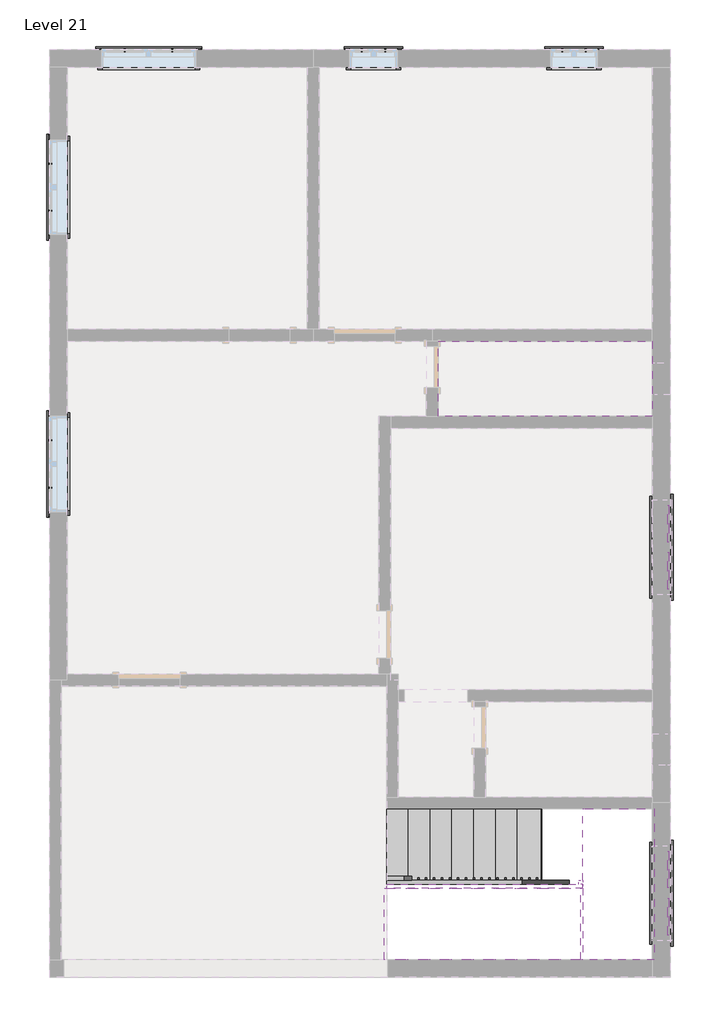
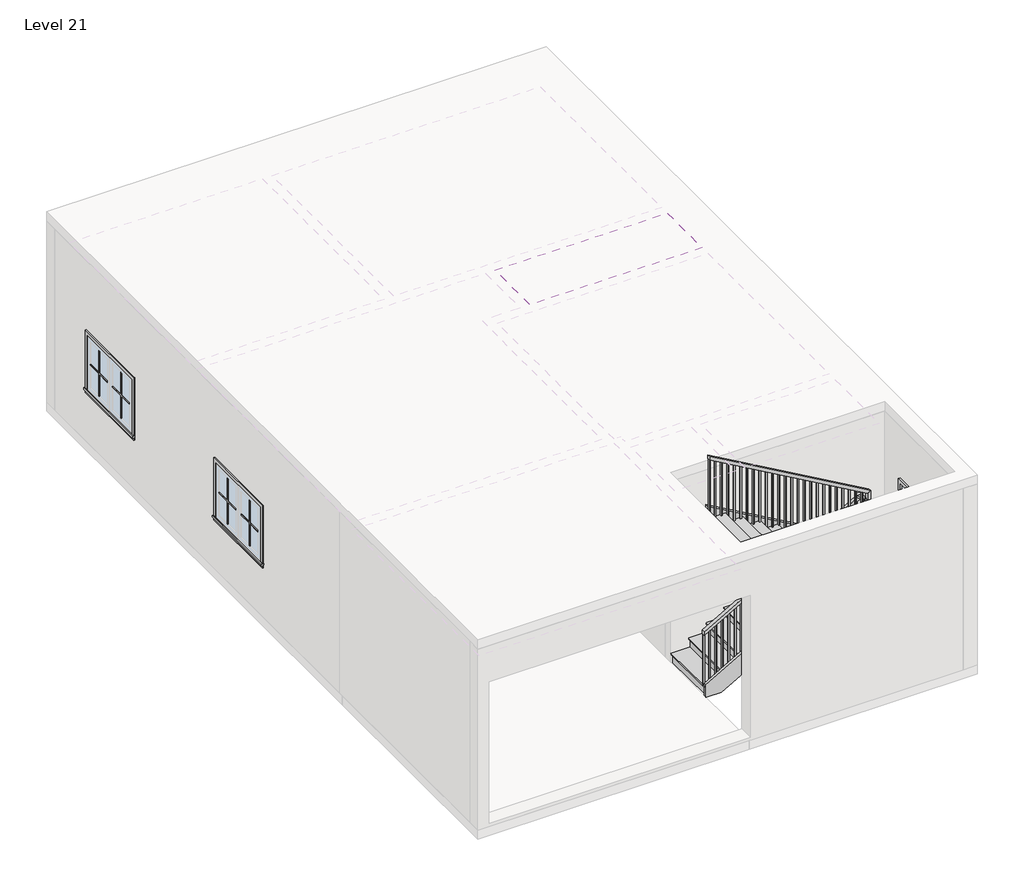
# One storey, part 2 of 2: 44 proxies, 3 members, 2 stair flights, 1 covering, 1 railing, 1 slab.
"""IFC4 building model written with IfcOpenShell, lengths in millimetres."""

from ifc_helpers import new_model, si_unit, frame, origin, place, context, project, spatial, polyline, outline, extrude, faceted_brep, transform, mapped, element, save
from components import muntin_pattern_2x2_muntin_pattern_2x2_2357e71d, muntin_pattern_2x2_muntin_pattern_2x2_302d8f29, muntin_pattern_2x2_muntin_pattern_2x2_53152e2c, muntin_pattern_2x2_muntin_pattern_2x2_e8f3e573, trim_window_exterior_flat_with_sill_c4e67c73, trim_window_exterior_flat_with_sill_a665a915, trim_window_interior_flat_picture_frame_cf1733af, trim_window_interior_flat_picture_frame_d485c387, non_monolithic_landing_5db28acc, stair_flight_6ff81285, stair_flight_de92f90a

model = new_model("IFC4")

# Units and contexts
model_context = context("Model", 3, world=origin())
ifc_project = project(units=[si_unit("LENGTHUNIT", "METRE", prefix="MILLI")], contexts=[model_context])

# Site, building, storey
site = spatial("IfcSite", under=ifc_project)
building = spatial("IfcBuilding", under=site)
storey = spatial("IfcBuildingStorey", under=building, Name="Level 21", Elevation=16002.0)

# Proxies
placement = place(None, origin())
muntin_pattern_2x2_muntin_pattern_2x2_shape = muntin_pattern_2x2_muntin_pattern_2x2_2357e71d(model_context)
element("IfcBuildingElementProxy", 1, Name="Muntin Pattern_2x2 : Muntin Pattern_2x2", ObjectType="Muntin Pattern_2x2 : Muntin Pattern_2x2", at=placement, inside=storey, context=model_context, shape_type="MappedRepresentation", body=[
    mapped(muntin_pattern_2x2_muntin_pattern_2x2_shape, transform((-4942.3279463, 5897.3080275, 16986.25), x_axis=(1.0, 0.0, 0.0), y_axis=(0.0, 1.0, 0.0), z_axis=(0.0, 0.0, 1.0))),
])
element("IfcBuildingElementProxy", 2, Name="Muntin Pattern_2x2 : Muntin Pattern_2x2", ObjectType="Muntin Pattern_2x2 : Muntin Pattern_2x2", at=placement, inside=storey, context=model_context, shape_type="MappedRepresentation", body=[
    mapped(muntin_pattern_2x2_muntin_pattern_2x2_shape, transform((-5899.5904463, 3838.3205275, 16986.25), x_axis=(0.0, 1.0, 0.0), y_axis=(-1.0, 0.0, 0.0), z_axis=(0.0, 0.0, 1.0))),
])
element("IfcBuildingElementProxy", 3, Name="Muntin Pattern_2x2 : Muntin Pattern_2x2", ObjectType="Muntin Pattern_2x2 : Muntin Pattern_2x2", at=placement, inside=storey, context=model_context, shape_type="MappedRepresentation", body=[
    mapped(muntin_pattern_2x2_muntin_pattern_2x2_shape, transform((-5899.5904463, 293.4330275, 16986.25), x_axis=(0.0, 1.0, 0.0), y_axis=(-1.0, 0.0, 0.0), z_axis=(0.0, 0.0, 1.0))),
])
element("IfcBuildingElementProxy", 4, Name="Muntin Pattern_2x2 : Muntin Pattern_2x2", ObjectType="Muntin Pattern_2x2 : Muntin Pattern_2x2", at=placement, inside=storey, context=model_context, shape_type="MappedRepresentation", body=[
    mapped(muntin_pattern_2x2_muntin_pattern_2x2_shape, transform((2031.5595537, -166.9419725, 17291.05), x_axis=(0.0, -1.0, 0.0), y_axis=(1.0, 0.0, 0.0), z_axis=(0.0, 0.0, 1.0))),
])
element("IfcBuildingElementProxy", 5, Name="Muntin Pattern_2x2 : Muntin Pattern_2x2", ObjectType="Muntin Pattern_2x2 : Muntin Pattern_2x2", at=placement, inside=storey, context=model_context, shape_type="MappedRepresentation", body=[
    mapped(muntin_pattern_2x2_muntin_pattern_2x2_shape, transform((2031.5595537, -4599.2419725, 17291.05), x_axis=(0.0, -1.0, 0.0), y_axis=(1.0, 0.0, 0.0), z_axis=(0.0, 0.0, 1.0))),
])
element("IfcBuildingElementProxy", 6, Name="Muntin Pattern_2x2 : Muntin Pattern_2x2", ObjectType="Muntin Pattern_2x2 : Muntin Pattern_2x2", at=placement, inside=storey, context=model_context, shape_type="MappedRepresentation", body=[
    mapped(muntin_pattern_2x2_muntin_pattern_2x2_shape, transform((-4942.3279463, 5897.3080275, 16986.25), x_axis=(1.0, 0.0, 0.0), y_axis=(0.0, 1.0, 0.0), z_axis=(0.0, 0.0, 1.0))),
])
element("IfcBuildingElementProxy", 7, Name="Muntin Pattern_2x2 : Muntin Pattern_2x2", ObjectType="Muntin Pattern_2x2 : Muntin Pattern_2x2", at=placement, inside=storey, context=model_context, shape_type="MappedRepresentation", body=[
    mapped(muntin_pattern_2x2_muntin_pattern_2x2_shape, transform((2031.5595537, -4599.2419725, 17291.05), x_axis=(0.0, -1.0, 0.0), y_axis=(1.0, 0.0, 0.0), z_axis=(0.0, 0.0, 1.0))),
])
muntin_pattern_2x2_muntin_pattern_2x2_2_shape = muntin_pattern_2x2_muntin_pattern_2x2_302d8f29(model_context)
element("IfcBuildingElementProxy", 8, Name="Muntin Pattern_2x2 : Muntin Pattern_2x2", ObjectType="Muntin Pattern_2x2 : Muntin Pattern_2x2", at=placement, inside=storey, context=model_context, shape_type="MappedRepresentation", body=[
    mapped(muntin_pattern_2x2_muntin_pattern_2x2_2_shape, transform((-4335.9029463, 5897.3080275, 16986.25), x_axis=(-1.0, 0.0, 0.0), y_axis=(0.0, -1.0, 0.0), z_axis=(0.0, 0.0, 1.0))),
])
element("IfcBuildingElementProxy", 9, Name="Muntin Pattern_2x2 : Muntin Pattern_2x2", ObjectType="Muntin Pattern_2x2 : Muntin Pattern_2x2", at=placement, inside=storey, context=model_context, shape_type="MappedRepresentation", body=[
    mapped(muntin_pattern_2x2_muntin_pattern_2x2_2_shape, transform((-5899.5904463, 4444.7455275, 16986.25), x_axis=(0.0, -1.0, 0.0), y_axis=(1.0, 0.0, 0.0), z_axis=(0.0, 0.0, 1.0))),
])
element("IfcBuildingElementProxy", 10, Name="Muntin Pattern_2x2 : Muntin Pattern_2x2", ObjectType="Muntin Pattern_2x2 : Muntin Pattern_2x2", at=placement, inside=storey, context=model_context, shape_type="MappedRepresentation", body=[
    mapped(muntin_pattern_2x2_muntin_pattern_2x2_2_shape, transform((-5899.5904463, 899.8580275, 16986.25), x_axis=(0.0, -1.0, 0.0), y_axis=(1.0, 0.0, 0.0), z_axis=(0.0, 0.0, 1.0))),
])
element("IfcBuildingElementProxy", 11, Name="Muntin Pattern_2x2 : Muntin Pattern_2x2", ObjectType="Muntin Pattern_2x2 : Muntin Pattern_2x2", at=placement, inside=storey, context=model_context, shape_type="MappedRepresentation", body=[
    mapped(muntin_pattern_2x2_muntin_pattern_2x2_2_shape, transform((2031.5595537, -773.3669725, 17291.05), x_axis=(0.0, 1.0, 0.0), y_axis=(-1.0, 0.0, 0.0), z_axis=(0.0, 0.0, 1.0))),
])
element("IfcBuildingElementProxy", 12, Name="Muntin Pattern_2x2 : Muntin Pattern_2x2", ObjectType="Muntin Pattern_2x2 : Muntin Pattern_2x2", at=placement, inside=storey, context=model_context, shape_type="MappedRepresentation", body=[
    mapped(muntin_pattern_2x2_muntin_pattern_2x2_2_shape, transform((2031.5595537, -5205.6669725, 17291.05), x_axis=(0.0, 1.0, 0.0), y_axis=(-1.0, 0.0, 0.0), z_axis=(0.0, 0.0, 1.0))),
])
element("IfcBuildingElementProxy", 13, Name="Muntin Pattern_2x2 : Muntin Pattern_2x2", ObjectType="Muntin Pattern_2x2 : Muntin Pattern_2x2", at=placement, inside=storey, context=model_context, shape_type="MappedRepresentation", body=[
    mapped(muntin_pattern_2x2_muntin_pattern_2x2_2_shape, transform((-4335.9029463, 5897.3080275, 16986.25), x_axis=(-1.0, 0.0, 0.0), y_axis=(0.0, -1.0, 0.0), z_axis=(0.0, 0.0, 1.0))),
])
element("IfcBuildingElementProxy", 14, Name="Muntin Pattern_2x2 : Muntin Pattern_2x2", ObjectType="Muntin Pattern_2x2 : Muntin Pattern_2x2", at=placement, inside=storey, context=model_context, shape_type="MappedRepresentation", body=[
    mapped(muntin_pattern_2x2_muntin_pattern_2x2_2_shape, transform((2031.5595537, -5205.6669725, 17291.05), x_axis=(0.0, 1.0, 0.0), y_axis=(-1.0, 0.0, 0.0), z_axis=(0.0, 0.0, 1.0))),
])
muntin_pattern_2x2_muntin_pattern_2x2_3_shape = muntin_pattern_2x2_muntin_pattern_2x2_53152e2c(model_context)
element("IfcBuildingElementProxy", 15, Name="Muntin Pattern_2x2 : Muntin Pattern_2x2", ObjectType="Muntin Pattern_2x2 : Muntin Pattern_2x2", at=placement, inside=storey, context=model_context, shape_type="MappedRepresentation", body=[
    mapped(muntin_pattern_2x2_muntin_pattern_2x2_3_shape, transform((-1907.0279463, 5897.3080275, 16986.25), x_axis=(1.0, 0.0, 0.0), y_axis=(0.0, 1.0, 0.0), z_axis=(0.0, 0.0, 1.0))),
])
element("IfcBuildingElementProxy", 16, Name="Muntin Pattern_2x2 : Muntin Pattern_2x2", ObjectType="Muntin Pattern_2x2 : Muntin Pattern_2x2", at=placement, inside=storey, context=model_context, shape_type="MappedRepresentation", body=[
    mapped(muntin_pattern_2x2_muntin_pattern_2x2_3_shape, transform((658.3720537, 5897.3080275, 16986.25), x_axis=(1.0, 0.0, 0.0), y_axis=(0.0, 1.0, 0.0), z_axis=(0.0, 0.0, 1.0))),
])
element("IfcBuildingElementProxy", 17, Name="Muntin Pattern_2x2 : Muntin Pattern_2x2", ObjectType="Muntin Pattern_2x2 : Muntin Pattern_2x2", at=placement, inside=storey, context=model_context, shape_type="MappedRepresentation", body=[
    mapped(muntin_pattern_2x2_muntin_pattern_2x2_3_shape, transform((-1907.0279463, 5897.3080275, 16986.25), x_axis=(1.0, 0.0, 0.0), y_axis=(0.0, 1.0, 0.0), z_axis=(0.0, 0.0, 1.0))),
])
element("IfcBuildingElementProxy", 18, Name="Muntin Pattern_2x2 : Muntin Pattern_2x2", ObjectType="Muntin Pattern_2x2 : Muntin Pattern_2x2", at=placement, inside=storey, context=model_context, shape_type="MappedRepresentation", body=[
    mapped(muntin_pattern_2x2_muntin_pattern_2x2_3_shape, transform((658.3720537, 5897.3080275, 16986.25), x_axis=(1.0, 0.0, 0.0), y_axis=(0.0, 1.0, 0.0), z_axis=(0.0, 0.0, 1.0))),
])
muntin_pattern_2x2_muntin_pattern_2x2_4_shape = muntin_pattern_2x2_muntin_pattern_2x2_e8f3e573(model_context)
element("IfcBuildingElementProxy", 19, Name="Muntin Pattern_2x2 : Muntin Pattern_2x2", ObjectType="Muntin Pattern_2x2 : Muntin Pattern_2x2", at=placement, inside=storey, context=model_context, shape_type="MappedRepresentation", body=[
    mapped(muntin_pattern_2x2_muntin_pattern_2x2_4_shape, transform((-1605.4029463, 5897.3080275, 16986.25), x_axis=(-1.0, 0.0, 0.0), y_axis=(0.0, -1.0, 0.0), z_axis=(0.0, 0.0, 1.0))),
])
element("IfcBuildingElementProxy", 20, Name="Muntin Pattern_2x2 : Muntin Pattern_2x2", ObjectType="Muntin Pattern_2x2 : Muntin Pattern_2x2", at=placement, inside=storey, context=model_context, shape_type="MappedRepresentation", body=[
    mapped(muntin_pattern_2x2_muntin_pattern_2x2_4_shape, transform((959.9970537, 5897.3080275, 16986.25), x_axis=(-1.0, 0.0, 0.0), y_axis=(0.0, -1.0, 0.0), z_axis=(0.0, 0.0, 1.0))),
])
element("IfcBuildingElementProxy", 21, Name="Muntin Pattern_2x2 : Muntin Pattern_2x2", ObjectType="Muntin Pattern_2x2 : Muntin Pattern_2x2", at=placement, inside=storey, context=model_context, shape_type="MappedRepresentation", body=[
    mapped(muntin_pattern_2x2_muntin_pattern_2x2_4_shape, transform((-1605.4029463, 5897.3080275, 16986.25), x_axis=(-1.0, 0.0, 0.0), y_axis=(0.0, -1.0, 0.0), z_axis=(0.0, 0.0, 1.0))),
])
element("IfcBuildingElementProxy", 22, Name="Muntin Pattern_2x2 : Muntin Pattern_2x2", ObjectType="Muntin Pattern_2x2 : Muntin Pattern_2x2", at=placement, inside=storey, context=model_context, shape_type="MappedRepresentation", body=[
    mapped(muntin_pattern_2x2_muntin_pattern_2x2_4_shape, transform((959.9970537, 5897.3080275, 16986.25), x_axis=(-1.0, 0.0, 0.0), y_axis=(0.0, -1.0, 0.0), z_axis=(0.0, 0.0, 1.0))),
])
trim_window_exterior_flat_with_sill_shape = trim_window_exterior_flat_with_sill_c4e67c73(model_context)
element("IfcBuildingElementProxy", 23, Name="Trim-Window-Exterior-Flat : with Sill", ObjectType="Trim-Window-Exterior-Flat : with Sill", at=placement, inside=storey, context=model_context, shape_type="MappedRepresentation", body=[
    mapped(trim_window_exterior_flat_with_sill_shape, transform((-4639.1154463, 5906.8330275, 17830.8), x_axis=(-1.0, 0.0, 0.0), y_axis=(0.0, 0.0, 1.0), z_axis=(0.0, 1.0, 0.0))),
])
element("IfcBuildingElementProxy", 24, Name="Trim-Window-Exterior-Flat : with Sill", ObjectType="Trim-Window-Exterior-Flat : with Sill", at=placement, inside=storey, context=model_context, shape_type="MappedRepresentation", body=[
    mapped(trim_window_exterior_flat_with_sill_shape, transform((-5909.1154463, 4141.5330275, 17830.8), x_axis=(0.0, -1.0, 0.0), y_axis=(0.0, 0.0, 1.0), z_axis=(-1.0, 0.0, 0.0))),
])
element("IfcBuildingElementProxy", 25, Name="Trim-Window-Exterior-Flat : with Sill", ObjectType="Trim-Window-Exterior-Flat : with Sill", at=placement, inside=storey, context=model_context, shape_type="MappedRepresentation", body=[
    mapped(trim_window_exterior_flat_with_sill_shape, transform((-5909.1154463, 596.6455275, 17830.8), x_axis=(0.0, -1.0, 0.0), y_axis=(0.0, 0.0, 1.0), z_axis=(-1.0, 0.0, 0.0))),
])
element("IfcBuildingElementProxy", 26, Name="Trim-Window-Exterior-Flat : with Sill", ObjectType="Trim-Window-Exterior-Flat : with Sill", at=placement, inside=storey, context=model_context, shape_type="MappedRepresentation", body=[
    mapped(trim_window_exterior_flat_with_sill_shape, transform((2041.0845537, -470.1544725, 18135.6), x_axis=(0.0, 1.0, 0.0), y_axis=(0.0, 0.0, 1.0), z_axis=(1.0, 0.0, 0.0))),
])
element("IfcBuildingElementProxy", 27, Name="Trim-Window-Exterior-Flat : with Sill", ObjectType="Trim-Window-Exterior-Flat : with Sill", at=placement, inside=storey, context=model_context, shape_type="MappedRepresentation", body=[
    mapped(trim_window_exterior_flat_with_sill_shape, transform((2041.0845537, -4902.4544725, 18135.6), x_axis=(0.0, 1.0, 0.0), y_axis=(0.0, 0.0, 1.0), z_axis=(1.0, 0.0, 0.0))),
])
element("IfcBuildingElementProxy", 28, Name="Trim-Window-Exterior-Flat : with Sill", ObjectType="Trim-Window-Exterior-Flat : with Sill", at=placement, inside=storey, context=model_context, shape_type="MappedRepresentation", body=[
    mapped(trim_window_exterior_flat_with_sill_shape, transform((-4639.1154463, 5906.8330275, 17830.8), x_axis=(-1.0, 0.0, 0.0), y_axis=(0.0, 0.0, 1.0), z_axis=(0.0, 1.0, 0.0))),
])
element("IfcBuildingElementProxy", 29, Name="Trim-Window-Exterior-Flat : with Sill", ObjectType="Trim-Window-Exterior-Flat : with Sill", at=placement, inside=storey, context=model_context, shape_type="MappedRepresentation", body=[
    mapped(trim_window_exterior_flat_with_sill_shape, transform((2041.0845537, -4902.4544725, 18135.6), x_axis=(0.0, 1.0, 0.0), y_axis=(0.0, 0.0, 1.0), z_axis=(1.0, 0.0, 0.0))),
])
trim_window_exterior_flat_with_sill_2_shape = trim_window_exterior_flat_with_sill_a665a915(model_context)
element("IfcBuildingElementProxy", 30, Name="Trim-Window-Exterior-Flat : with Sill", ObjectType="Trim-Window-Exterior-Flat : with Sill", at=placement, inside=storey, context=model_context, shape_type="MappedRepresentation", body=[
    mapped(trim_window_exterior_flat_with_sill_2_shape, transform((-1756.2154463, 5906.8330275, 17830.8), x_axis=(-1.0, 0.0, 0.0), y_axis=(0.0, 0.0, 1.0), z_axis=(0.0, 1.0, 0.0))),
])
element("IfcBuildingElementProxy", 31, Name="Trim-Window-Exterior-Flat : with Sill", ObjectType="Trim-Window-Exterior-Flat : with Sill", at=placement, inside=storey, context=model_context, shape_type="MappedRepresentation", body=[
    mapped(trim_window_exterior_flat_with_sill_2_shape, transform((809.1845537, 5906.8330275, 17830.8), x_axis=(-1.0, 0.0, 0.0), y_axis=(0.0, 0.0, 1.0), z_axis=(0.0, 1.0, 0.0))),
])
element("IfcBuildingElementProxy", 32, Name="Trim-Window-Exterior-Flat : with Sill", ObjectType="Trim-Window-Exterior-Flat : with Sill", at=placement, inside=storey, context=model_context, shape_type="MappedRepresentation", body=[
    mapped(trim_window_exterior_flat_with_sill_2_shape, transform((-1756.2154463, 5906.8330275, 17830.8), x_axis=(-1.0, 0.0, 0.0), y_axis=(0.0, 0.0, 1.0), z_axis=(0.0, 1.0, 0.0))),
])
element("IfcBuildingElementProxy", 33, Name="Trim-Window-Exterior-Flat : with Sill", ObjectType="Trim-Window-Exterior-Flat : with Sill", at=placement, inside=storey, context=model_context, shape_type="MappedRepresentation", body=[
    mapped(trim_window_exterior_flat_with_sill_2_shape, transform((809.1845537, 5906.8330275, 17830.8), x_axis=(-1.0, 0.0, 0.0), y_axis=(0.0, 0.0, 1.0), z_axis=(0.0, 1.0, 0.0))),
])
trim_window_interior_flat_picture_frame_shape = trim_window_interior_flat_picture_frame_cf1733af(model_context)
element("IfcBuildingElementProxy", 34, Name="Trim-Window-Interior-Flat : Picture Frame", ObjectType="Trim-Window-Interior-Flat : Picture Frame", at=placement, inside=storey, context=model_context, shape_type="MappedRepresentation", body=[
    mapped(trim_window_interior_flat_picture_frame_shape, transform((-4639.1154463, 5678.2330275, 17830.8), x_axis=(1.0, 0.0, 0.0), y_axis=(0.0, 0.0, 1.0), z_axis=(0.0, -1.0, 0.0))),
])
element("IfcBuildingElementProxy", 35, Name="Trim-Window-Interior-Flat : Picture Frame", ObjectType="Trim-Window-Interior-Flat : Picture Frame", at=placement, inside=storey, context=model_context, shape_type="MappedRepresentation", body=[
    mapped(trim_window_interior_flat_picture_frame_shape, transform((-5680.5154463, 4141.5330275, 17830.8), x_axis=(0.0, 1.0, 0.0), y_axis=(0.0, 0.0, 1.0), z_axis=(1.0, 0.0, 0.0))),
])
element("IfcBuildingElementProxy", 36, Name="Trim-Window-Interior-Flat : Picture Frame", ObjectType="Trim-Window-Interior-Flat : Picture Frame", at=placement, inside=storey, context=model_context, shape_type="MappedRepresentation", body=[
    mapped(trim_window_interior_flat_picture_frame_shape, transform((-5680.5154463, 596.6455275, 17830.8), x_axis=(0.0, 1.0, 0.0), y_axis=(0.0, 0.0, 1.0), z_axis=(1.0, 0.0, 0.0))),
])
element("IfcBuildingElementProxy", 37, Name="Trim-Window-Interior-Flat : Picture Frame", ObjectType="Trim-Window-Interior-Flat : Picture Frame", at=placement, inside=storey, context=model_context, shape_type="MappedRepresentation", body=[
    mapped(trim_window_interior_flat_picture_frame_shape, transform((1812.4845537, -470.1544725, 18135.6), x_axis=(0.0, -1.0, 0.0), y_axis=(0.0, 0.0, 1.0), z_axis=(-1.0, 0.0, 0.0))),
])
element("IfcBuildingElementProxy", 38, Name="Trim-Window-Interior-Flat : Picture Frame", ObjectType="Trim-Window-Interior-Flat : Picture Frame", at=placement, inside=storey, context=model_context, shape_type="MappedRepresentation", body=[
    mapped(trim_window_interior_flat_picture_frame_shape, transform((1812.4845537, -4902.4544725, 18135.6), x_axis=(0.0, -1.0, 0.0), y_axis=(0.0, 0.0, 1.0), z_axis=(-1.0, 0.0, 0.0))),
])
element("IfcBuildingElementProxy", 39, Name="Trim-Window-Interior-Flat : Picture Frame", ObjectType="Trim-Window-Interior-Flat : Picture Frame", at=placement, inside=storey, context=model_context, shape_type="MappedRepresentation", body=[
    mapped(trim_window_interior_flat_picture_frame_shape, transform((-4639.1154463, 5678.2330275, 17830.8), x_axis=(1.0, 0.0, 0.0), y_axis=(0.0, 0.0, 1.0), z_axis=(0.0, -1.0, 0.0))),
])
element("IfcBuildingElementProxy", 40, Name="Trim-Window-Interior-Flat : Picture Frame", ObjectType="Trim-Window-Interior-Flat : Picture Frame", at=placement, inside=storey, context=model_context, shape_type="MappedRepresentation", body=[
    mapped(trim_window_interior_flat_picture_frame_shape, transform((1812.4845537, -4902.4544725, 18135.6), x_axis=(0.0, -1.0, 0.0), y_axis=(0.0, 0.0, 1.0), z_axis=(-1.0, 0.0, 0.0))),
])
trim_window_interior_flat_picture_frame_2_shape = trim_window_interior_flat_picture_frame_d485c387(model_context)
element("IfcBuildingElementProxy", 41, Name="Trim-Window-Interior-Flat : Picture Frame", ObjectType="Trim-Window-Interior-Flat : Picture Frame", at=placement, inside=storey, context=model_context, shape_type="MappedRepresentation", body=[
    mapped(trim_window_interior_flat_picture_frame_2_shape, transform((-1756.2154463, 5678.2330275, 17830.8), x_axis=(1.0, 0.0, 0.0), y_axis=(0.0, 0.0, 1.0), z_axis=(0.0, -1.0, 0.0))),
])
element("IfcBuildingElementProxy", 42, Name="Trim-Window-Interior-Flat : Picture Frame", ObjectType="Trim-Window-Interior-Flat : Picture Frame", at=placement, inside=storey, context=model_context, shape_type="MappedRepresentation", body=[
    mapped(trim_window_interior_flat_picture_frame_2_shape, transform((809.1845537, 5678.2330275, 17830.8), x_axis=(1.0, 0.0, 0.0), y_axis=(0.0, 0.0, 1.0), z_axis=(0.0, -1.0, 0.0))),
])
element("IfcBuildingElementProxy", 43, Name="Trim-Window-Interior-Flat : Picture Frame", ObjectType="Trim-Window-Interior-Flat : Picture Frame", at=placement, inside=storey, context=model_context, shape_type="MappedRepresentation", body=[
    mapped(trim_window_interior_flat_picture_frame_2_shape, transform((-1756.2154463, 5678.2330275, 17830.8), x_axis=(1.0, 0.0, 0.0), y_axis=(0.0, 0.0, 1.0), z_axis=(0.0, -1.0, 0.0))),
])
element("IfcBuildingElementProxy", 44, Name="Trim-Window-Interior-Flat : Picture Frame", ObjectType="Trim-Window-Interior-Flat : Picture Frame", at=placement, inside=storey, context=model_context, shape_type="MappedRepresentation", body=[
    mapped(trim_window_interior_flat_picture_frame_2_shape, transform((809.1845537, 5678.2330275, 17830.8), x_axis=(1.0, 0.0, 0.0), y_axis=(0.0, 0.0, 1.0), z_axis=(0.0, -1.0, 0.0))),
])

# Covering
element("IfcCovering", 45, ObjectType="2' x 4' ACT System", at=placement, inside=storey, context=model_context, shape_type="SweptSolid", body=[
    extrude(outline(polyline([(-930.7154463, 2171.4455275), (1812.4845537, 2171.4455275), (1812.4845537, 1206.2455275), (-930.7154463, 1206.2455275), (-930.7154463, 2171.4455275)])), frame((0.0, 0.0, 18745.2), z_axis=(0.0, 0.0, 1.0), x_axis=(1.0, 0.0, 0.0)), (0.0, 0.0, 1.0), 57.15),
])

# Members
element("IfcMember", 46, ObjectType="Stringer - 2\" Width", at=placement, inside=storey, context=model_context, shape_type="SweptSolid", body=[
    extrude(outline(polyline([(16211.0890626, -1591.1154463), (16002.0, -1591.1154463), (16002.0, -1342.8974141), (17270.924218, 872.6845537), (17622.1745172, 872.6845537), (16211.0890626, -1591.1154463)])), frame((0.0, -4788.1544725, 0.0), z_axis=(0.0, 1.0, 0.0), x_axis=(0.0, 0.0, 1.0)), (0.0, 0.0, 1.0), 50.8),
])
element("IfcMember", 47, ObjectType="Stringer - 2\" Width", at=placement, inside=storey, context=model_context, shape_type="SweptSolid", body=[
    extrude(outline(polyline([(17460.0387634, 923.4845537), (17811.2890626, 923.4845537), (19251.4690626, -1591.1154463), (18900.2187634, -1591.1154463), (17460.0387634, 923.4845537)])), frame((0.0, -4838.9544725, 0.0), z_axis=(0.0, 1.0, 0.0), x_axis=(0.0, 0.0, 1.0)), (0.0, 0.0, 1.0), 50.8),
])
element("IfcMember", 48, ObjectType="Stringer - 2\" Width", at=placement, inside=storey, context=model_context, shape_type="SweptSolid", body=[
    extrude(outline(polyline([(872.6845537, -4737.3544725), (923.4845537, -4737.3544725), (923.4845537, -4788.1544725), (872.6845537, -4788.1544725), (872.6845537, -4737.3544725)])), frame((0.0, 0.0, 17373.6), z_axis=(0.0, 0.0, 1.0), x_axis=(1.0, 0.0, 0.0)), (0.0, 0.0, 1.0), 304.8),
])

# Railing
element("IfcRailing", 49, ObjectType="Handrail - Rectangular", at=placement, inside=storey, context=model_context, shape_type="SolidModel", body=[
    faceted_brep([(-1591.1154463, -4686.5544725, 17076.42), (-1591.1154463, -4686.5544725, 17017.8782835), (-1591.1154463, -4737.3544725, 17017.8782835), (-1591.1154463, -4737.3544725, 17076.42), (847.2845537, -4686.5544725, 18472.9581818), (898.0845537, -4686.5544725, 18443.5110107), (898.0845537, -4737.3544725, 18443.5110107), (847.2845537, -4737.3544725, 18472.9581818), (847.2845537, -4686.5544725, 18516.6), (898.0845537, -4686.5544725, 18465.8), (898.0845537, -4737.3544725, 18465.8), (847.2845537, -4737.3544725, 18516.6), (974.2845537, -4686.5544725, 18516.6), (974.2845537, -4686.5544725, 18465.8), (923.4845537, -4737.3544725, 18465.8), (923.4845537, -4737.3544725, 18516.6), (974.2845537, -4813.5544725, 18516.6), (974.2845537, -4813.5544725, 18465.8), (923.4845537, -4813.5544725, 18465.8), (923.4845537, -4813.5544725, 18516.6), (974.2845537, -4838.9544725, 18516.6), (923.4845537, -4838.9544725, 18516.6), (923.4845537, -4889.7544725, 18465.8), (974.2845537, -4889.7544725, 18465.8)], [[[0, 1, 2, 3]], [[1, 0, 4, 5]], [[2, 1, 5, 6]], [[3, 2, 6, 7]], [[0, 3, 7, 4]], [[5, 4, 8, 9]], [[6, 5, 9, 10]], [[7, 6, 10, 11]], [[4, 7, 11, 8]], [[9, 8, 12, 13]], [[10, 9, 13, 14]], [[11, 10, 14, 15]], [[8, 11, 15, 12]], [[13, 12, 16, 17]], [[14, 13, 17, 18]], [[15, 14, 18, 19]], [[12, 15, 19, 16]], [[20, 21, 22, 23]], [[17, 16, 20, 23]], [[18, 17, 23, 22]], [[19, 18, 22, 21]], [[16, 19, 21, 20]]]),
    faceted_brep([(974.2845537, -4838.9544725, 18516.6), (974.2845537, -4889.7544725, 18465.8), (923.4845537, -4889.7544725, 18465.8), (923.4845537, -4838.9544725, 18516.6), (974.2845537, -4838.9544725, 18647.5254545), (923.4845537, -4838.9544725, 18618.0782835), (923.4845537, -4889.7544725, 18618.0782835), (974.2845537, -4889.7544725, 18647.5254545)], [[[0, 1, 2, 3]], [[4, 5, 6, 7]], [[1, 0, 4, 7]], [[2, 1, 7, 6]], [[3, 2, 6, 5]], [[0, 3, 5, 4]]]),
    faceted_brep([(974.2845537, -4889.7544725, 18647.5254545), (923.4845537, -4889.7544725, 18618.0782835), (923.4845537, -4838.9544725, 18618.0782835), (974.2845537, -4838.9544725, 18647.5254545), (-1591.1154463, -4889.7544725, 20116.8), (-1591.1154463, -4838.9544725, 20116.8), (-1591.1154463, -4838.9544725, 20058.2582835), (-1591.1154463, -4889.7544725, 20058.2582835)], [[[0, 1, 2, 3]], [[4, 5, 6, 7]], [[1, 0, 4, 7]], [[2, 1, 7, 6]], [[3, 2, 6, 5]], [[0, 3, 5, 4]]]),
    extrude(outline(polyline([(19994.6139653, -1479.9904463), (20005.5244198, -1499.0404463), (19042.38, -1499.0404463), (19042.38, -1479.9904463), (19994.6139653, -1479.9904463)])), frame((0.0, -4873.8794725, 0.0), z_axis=(0.0, 1.0, 0.0), x_axis=(0.0, 0.0, 1.0)), (0.0, 0.0, 1.0), 19.05),
    extrude(outline(polyline([(19936.4248744, -1378.3904463), (19947.3353289, -1397.4404463), (19042.38, -1397.4404463), (19042.38, -1378.3904463), (19936.4248744, -1378.3904463)])), frame((0.0, -4873.8794725, 0.0), z_axis=(0.0, 1.0, 0.0), x_axis=(0.0, 0.0, 1.0)), (0.0, 0.0, 1.0), 19.05),
    extrude(outline(polyline([(19878.2357835, -1276.7904463), (19889.146238, -1295.8404463), (18882.36, -1295.8404463), (18882.36, -1276.7904463), (19878.2357835, -1276.7904463)])), frame((0.0, -4873.8794725, 0.0), z_axis=(0.0, 1.0, 0.0), x_axis=(0.0, 0.0, 1.0)), (0.0, 0.0, 1.0), 19.05),
    extrude(outline(polyline([(19820.0466926, -1175.1904463), (19830.9571471, -1194.2404463), (18882.36, -1194.2404463), (18882.36, -1175.1904463), (19820.0466926, -1175.1904463)])), frame((0.0, -4873.8794725, 0.0), z_axis=(0.0, 1.0, 0.0), x_axis=(0.0, 0.0, 1.0)), (0.0, 0.0, 1.0), 19.05),
    extrude(outline(polyline([(19761.8576016, -1073.5904463), (19772.7680562, -1092.6404463), (18882.36, -1092.6404463), (18882.36, -1073.5904463), (19761.8576016, -1073.5904463)])), frame((0.0, -4873.8794725, 0.0), z_axis=(0.0, 1.0, 0.0), x_axis=(0.0, 0.0, 1.0)), (0.0, 0.0, 1.0), 19.05),
    extrude(outline(polyline([(19703.6685107, -971.9904463), (19714.5789653, -991.0404463), (18722.34, -991.0404463), (18722.34, -971.9904463), (19703.6685107, -971.9904463)])), frame((0.0, -4873.8794725, 0.0), z_axis=(0.0, 1.0, 0.0), x_axis=(0.0, 0.0, 1.0)), (0.0, 0.0, 1.0), 19.05),
    extrude(outline(polyline([(19645.4794198, -870.3904463), (19656.3898744, -889.4404463), (18722.34, -889.4404463), (18722.34, -870.3904463), (19645.4794198, -870.3904463)])), frame((0.0, -4873.8794725, 0.0), z_axis=(0.0, 1.0, 0.0), x_axis=(0.0, 0.0, 1.0)), (0.0, 0.0, 1.0), 19.05),
    extrude(outline(polyline([(19587.2903289, -768.7904463), (19598.2007835, -787.8404463), (18722.34, -787.8404463), (18722.34, -768.7904463), (19587.2903289, -768.7904463)])), frame((0.0, -4873.8794725, 0.0), z_axis=(0.0, 1.0, 0.0), x_axis=(0.0, 0.0, 1.0)), (0.0, 0.0, 1.0), 19.05),
    extrude(outline(polyline([(19529.101238, -667.1904463), (19540.0116926, -686.2404463), (18562.32, -686.2404463), (18562.32, -667.1904463), (19529.101238, -667.1904463)])), frame((0.0, -4873.8794725, 0.0), z_axis=(0.0, 1.0, 0.0), x_axis=(0.0, 0.0, 1.0)), (0.0, 0.0, 1.0), 19.05),
    extrude(outline(polyline([(19470.9121471, -565.5904463), (19481.8226016, -584.6404463), (18562.32, -584.6404463), (18562.32, -565.5904463), (19470.9121471, -565.5904463)])), frame((0.0, -4873.8794725, 0.0), z_axis=(0.0, 1.0, 0.0), x_axis=(0.0, 0.0, 1.0)), (0.0, 0.0, 1.0), 19.05),
    extrude(outline(polyline([(19412.7230562, -463.9904463), (19423.6335107, -483.0404463), (18562.32, -483.0404463), (18562.32, -463.9904463), (19412.7230562, -463.9904463)])), frame((0.0, -4873.8794725, 0.0), z_axis=(0.0, 1.0, 0.0), x_axis=(0.0, 0.0, 1.0)), (0.0, 0.0, 1.0), 19.05),
    extrude(outline(polyline([(19354.5339653, -362.3904463), (19365.4444198, -381.4404463), (18402.3, -381.4404463), (18402.3, -362.3904463), (19354.5339653, -362.3904463)])), frame((0.0, -4873.8794725, 0.0), z_axis=(0.0, 1.0, 0.0), x_axis=(0.0, 0.0, 1.0)), (0.0, 0.0, 1.0), 19.05),
    extrude(outline(polyline([(19296.3448744, -260.7904463), (19307.2553289, -279.8404463), (18402.3, -279.8404463), (18402.3, -260.7904463), (19296.3448744, -260.7904463)])), frame((0.0, -4873.8794725, 0.0), z_axis=(0.0, 1.0, 0.0), x_axis=(0.0, 0.0, 1.0)), (0.0, 0.0, 1.0), 19.05),
    extrude(outline(polyline([(19238.1557835, -159.1904463), (19249.066238, -178.2404463), (18242.28, -178.2404463), (18242.28, -159.1904463), (19238.1557835, -159.1904463)])), frame((0.0, -4873.8794725, 0.0), z_axis=(0.0, 1.0, 0.0), x_axis=(0.0, 0.0, 1.0)), (0.0, 0.0, 1.0), 19.05),
    extrude(outline(polyline([(19179.9666926, -57.5904463), (19190.8771471, -76.6404463), (18242.28, -76.6404463), (18242.28, -57.5904463), (19179.9666926, -57.5904463)])), frame((0.0, -4873.8794725, 0.0), z_axis=(0.0, 1.0, 0.0), x_axis=(0.0, 0.0, 1.0)), (0.0, 0.0, 1.0), 19.05),
    extrude(outline(polyline([(19121.7776016, 44.0095537), (19132.6880562, 24.9595537), (18242.28, 24.9595537), (18242.28, 44.0095537), (19121.7776016, 44.0095537)])), frame((0.0, -4873.8794725, 0.0), z_axis=(0.0, 1.0, 0.0), x_axis=(0.0, 0.0, 1.0)), (0.0, 0.0, 1.0), 19.05),
    extrude(outline(polyline([(19063.5885107, 145.6095537), (19074.4989653, 126.5595537), (18082.26, 126.5595537), (18082.26, 145.6095537), (19063.5885107, 145.6095537)])), frame((0.0, -4873.8794725, 0.0), z_axis=(0.0, 1.0, 0.0), x_axis=(0.0, 0.0, 1.0)), (0.0, 0.0, 1.0), 19.05),
    extrude(outline(polyline([(19005.3994198, 247.2095537), (19016.3098744, 228.1595537), (18082.26, 228.1595537), (18082.26, 247.2095537), (19005.3994198, 247.2095537)])), frame((0.0, -4873.8794725, 0.0), z_axis=(0.0, 1.0, 0.0), x_axis=(0.0, 0.0, 1.0)), (0.0, 0.0, 1.0), 19.05),
    extrude(outline(polyline([(18947.2103289, 348.8095537), (18958.1207835, 329.7595537), (18082.26, 329.7595537), (18082.26, 348.8095537), (18947.2103289, 348.8095537)])), frame((0.0, -4873.8794725, 0.0), z_axis=(0.0, 1.0, 0.0), x_axis=(0.0, 0.0, 1.0)), (0.0, 0.0, 1.0), 19.05),
    extrude(outline(polyline([(18889.021238, 450.4095537), (18899.9316926, 431.3595537), (17922.24, 431.3595537), (17922.24, 450.4095537), (18889.021238, 450.4095537)])), frame((0.0, -4873.8794725, 0.0), z_axis=(0.0, 1.0, 0.0), x_axis=(0.0, 0.0, 1.0)), (0.0, 0.0, 1.0), 19.05),
    extrude(outline(polyline([(18830.8321471, 552.0095537), (18841.7426016, 532.9595537), (17922.24, 532.9595537), (17922.24, 552.0095537), (18830.8321471, 552.0095537)])), frame((0.0, -4873.8794725, 0.0), z_axis=(0.0, 1.0, 0.0), x_axis=(0.0, 0.0, 1.0)), (0.0, 0.0, 1.0), 19.05),
    extrude(outline(polyline([(18772.6430562, 653.6095537), (18783.5535107, 634.5595537), (17922.24, 634.5595537), (17922.24, 653.6095537), (18772.6430562, 653.6095537)])), frame((0.0, -4873.8794725, 0.0), z_axis=(0.0, 1.0, 0.0), x_axis=(0.0, 0.0, 1.0)), (0.0, 0.0, 1.0), 19.05),
    extrude(outline(polyline([(18714.4539653, 755.2095537), (18725.3644198, 736.1595537), (17762.22, 736.1595537), (17762.22, 755.2095537), (18714.4539653, 755.2095537)])), frame((0.0, -4873.8794725, 0.0), z_axis=(0.0, 1.0, 0.0), x_axis=(0.0, 0.0, 1.0)), (0.0, 0.0, 1.0), 19.05),
    extrude(outline(polyline([(18656.2648744, 856.8095537), (18667.1753289, 837.7595537), (17762.22, 837.7595537), (17762.22, 856.8095537), (18656.2648744, 856.8095537)])), frame((0.0, -4873.8794725, 0.0), z_axis=(0.0, 1.0, 0.0), x_axis=(0.0, 0.0, 1.0)), (0.0, 0.0, 1.0), 19.05),
    extrude(outline(polyline([(939.3595537, -4804.0294725), (958.4095537, -4804.0294725), (958.4095537, -4823.0794725), (939.3595537, -4823.0794725), (939.3595537, -4804.0294725)])), frame((0.0, 0.0, 17602.2), z_axis=(0.0, 0.0, 1.0), x_axis=(1.0, 0.0, 0.0)), (0.0, 0.0, 1.0), 863.6),
    extrude(outline(polyline([(18419.8716926, 856.8095537), (18408.961238, 837.7595537), (17442.18, 837.7595537), (17442.18, 856.8095537), (18419.8716926, 856.8095537)])), frame((0.0, -4721.4794725, 0.0), z_axis=(0.0, 1.0, 0.0), x_axis=(0.0, 0.0, 1.0)), (0.0, 0.0, 1.0), 19.05),
    extrude(outline(polyline([(18361.6826016, 755.2095537), (18350.7721471, 736.1595537), (17442.18, 736.1595537), (17442.18, 755.2095537), (18361.6826016, 755.2095537)])), frame((0.0, -4721.4794725, 0.0), z_axis=(0.0, 1.0, 0.0), x_axis=(0.0, 0.0, 1.0)), (0.0, 0.0, 1.0), 19.05),
    extrude(outline(polyline([(18303.4935107, 653.6095537), (18292.5830562, 634.5595537), (17442.18, 634.5595537), (17442.18, 653.6095537), (18303.4935107, 653.6095537)])), frame((0.0, -4721.4794725, 0.0), z_axis=(0.0, 1.0, 0.0), x_axis=(0.0, 0.0, 1.0)), (0.0, 0.0, 1.0), 19.05),
    extrude(outline(polyline([(18245.3044198, 552.0095537), (18234.3939653, 532.9595537), (17282.16, 532.9595537), (17282.16, 552.0095537), (18245.3044198, 552.0095537)])), frame((0.0, -4721.4794725, 0.0), z_axis=(0.0, 1.0, 0.0), x_axis=(0.0, 0.0, 1.0)), (0.0, 0.0, 1.0), 19.05),
    extrude(outline(polyline([(18187.1153289, 450.4095537), (18176.2048744, 431.3595537), (17282.16, 431.3595537), (17282.16, 450.4095537), (18187.1153289, 450.4095537)])), frame((0.0, -4721.4794725, 0.0), z_axis=(0.0, 1.0, 0.0), x_axis=(0.0, 0.0, 1.0)), (0.0, 0.0, 1.0), 19.05),
    extrude(outline(polyline([(18128.926238, 348.8095537), (18118.0157835, 329.7595537), (17122.14, 329.7595537), (17122.14, 348.8095537), (18128.926238, 348.8095537)])), frame((0.0, -4721.4794725, 0.0), z_axis=(0.0, 1.0, 0.0), x_axis=(0.0, 0.0, 1.0)), (0.0, 0.0, 1.0), 19.05),
    extrude(outline(polyline([(18070.7371471, 247.2095537), (18059.8266926, 228.1595537), (17122.14, 228.1595537), (17122.14, 247.2095537), (18070.7371471, 247.2095537)])), frame((0.0, -4721.4794725, 0.0), z_axis=(0.0, 1.0, 0.0), x_axis=(0.0, 0.0, 1.0)), (0.0, 0.0, 1.0), 19.05),
    extrude(outline(polyline([(18012.5480562, 145.6095537), (18001.6376016, 126.5595537), (17122.14, 126.5595537), (17122.14, 145.6095537), (18012.5480562, 145.6095537)])), frame((0.0, -4721.4794725, 0.0), z_axis=(0.0, 1.0, 0.0), x_axis=(0.0, 0.0, 1.0)), (0.0, 0.0, 1.0), 19.05),
    extrude(outline(polyline([(17954.3589653, 44.0095537), (17943.4485107, 24.9595537), (16962.12, 24.9595537), (16962.12, 44.0095537), (17954.3589653, 44.0095537)])), frame((0.0, -4721.4794725, 0.0), z_axis=(0.0, 1.0, 0.0), x_axis=(0.0, 0.0, 1.0)), (0.0, 0.0, 1.0), 19.05),
    extrude(outline(polyline([(17896.1698744, -57.5904463), (17885.2594198, -76.6404463), (16962.12, -76.6404463), (16962.12, -57.5904463), (17896.1698744, -57.5904463)])), frame((0.0, -4721.4794725, 0.0), z_axis=(0.0, 1.0, 0.0), x_axis=(0.0, 0.0, 1.0)), (0.0, 0.0, 1.0), 19.05),
    extrude(outline(polyline([(17837.9807835, -159.1904463), (17827.0703289, -178.2404463), (16962.12, -178.2404463), (16962.12, -159.1904463), (17837.9807835, -159.1904463)])), frame((0.0, -4721.4794725, 0.0), z_axis=(0.0, 1.0, 0.0), x_axis=(0.0, 0.0, 1.0)), (0.0, 0.0, 1.0), 19.05),
    extrude(outline(polyline([(17779.7916926, -260.7904463), (17768.881238, -279.8404463), (16802.1, -279.8404463), (16802.1, -260.7904463), (17779.7916926, -260.7904463)])), frame((0.0, -4721.4794725, 0.0), z_axis=(0.0, 1.0, 0.0), x_axis=(0.0, 0.0, 1.0)), (0.0, 0.0, 1.0), 19.05),
    extrude(outline(polyline([(17721.6026016, -362.3904463), (17710.6921471, -381.4404463), (16802.1, -381.4404463), (16802.1, -362.3904463), (17721.6026016, -362.3904463)])), frame((0.0, -4721.4794725, 0.0), z_axis=(0.0, 1.0, 0.0), x_axis=(0.0, 0.0, 1.0)), (0.0, 0.0, 1.0), 19.05),
    extrude(outline(polyline([(17663.4135107, -463.9904463), (17652.5030562, -483.0404463), (16802.1, -483.0404463), (16802.1, -463.9904463), (17663.4135107, -463.9904463)])), frame((0.0, -4721.4794725, 0.0), z_axis=(0.0, 1.0, 0.0), x_axis=(0.0, 0.0, 1.0)), (0.0, 0.0, 1.0), 19.05),
    extrude(outline(polyline([(17605.2244198, -565.5904463), (17594.3139653, -584.6404463), (16642.08, -584.6404463), (16642.08, -565.5904463), (17605.2244198, -565.5904463)])), frame((0.0, -4721.4794725, 0.0), z_axis=(0.0, 1.0, 0.0), x_axis=(0.0, 0.0, 1.0)), (0.0, 0.0, 1.0), 19.05),
    extrude(outline(polyline([(17547.0353289, -667.1904463), (17536.1248744, -686.2404463), (16642.08, -686.2404463), (16642.08, -667.1904463), (17547.0353289, -667.1904463)])), frame((0.0, -4721.4794725, 0.0), z_axis=(0.0, 1.0, 0.0), x_axis=(0.0, 0.0, 1.0)), (0.0, 0.0, 1.0), 19.05),
    extrude(outline(polyline([(17488.846238, -768.7904463), (17477.9357835, -787.8404463), (16482.06, -787.8404463), (16482.06, -768.7904463), (17488.846238, -768.7904463)])), frame((0.0, -4721.4794725, 0.0), z_axis=(0.0, 1.0, 0.0), x_axis=(0.0, 0.0, 1.0)), (0.0, 0.0, 1.0), 19.05),
    extrude(outline(polyline([(17430.6571471, -870.3904463), (17419.7466926, -889.4404463), (16482.06, -889.4404463), (16482.06, -870.3904463), (17430.6571471, -870.3904463)])), frame((0.0, -4721.4794725, 0.0), z_axis=(0.0, 1.0, 0.0), x_axis=(0.0, 0.0, 1.0)), (0.0, 0.0, 1.0), 19.05),
    extrude(outline(polyline([(17372.4680562, -971.9904463), (17361.5576016, -991.0404463), (16482.06, -991.0404463), (16482.06, -971.9904463), (17372.4680562, -971.9904463)])), frame((0.0, -4721.4794725, 0.0), z_axis=(0.0, 1.0, 0.0), x_axis=(0.0, 0.0, 1.0)), (0.0, 0.0, 1.0), 19.05),
    extrude(outline(polyline([(17314.2789653, -1073.5904463), (17303.3685107, -1092.6404463), (16322.04, -1092.6404463), (16322.04, -1073.5904463), (17314.2789653, -1073.5904463)])), frame((0.0, -4721.4794725, 0.0), z_axis=(0.0, 1.0, 0.0), x_axis=(0.0, 0.0, 1.0)), (0.0, 0.0, 1.0), 19.05),
    extrude(outline(polyline([(17256.0898744, -1175.1904463), (17245.1794198, -1194.2404463), (16322.04, -1194.2404463), (16322.04, -1175.1904463), (17256.0898744, -1175.1904463)])), frame((0.0, -4721.4794725, 0.0), z_axis=(0.0, 1.0, 0.0), x_axis=(0.0, 0.0, 1.0)), (0.0, 0.0, 1.0), 19.05),
    extrude(outline(polyline([(17197.9007835, -1276.7904463), (17186.9903289, -1295.8404463), (16322.04, -1295.8404463), (16322.04, -1276.7904463), (17197.9007835, -1276.7904463)])), frame((0.0, -4721.4794725, 0.0), z_axis=(0.0, 1.0, 0.0), x_axis=(0.0, 0.0, 1.0)), (0.0, 0.0, 1.0), 19.05),
    extrude(outline(polyline([(17139.7116926, -1378.3904463), (17128.801238, -1397.4404463), (16162.02, -1397.4404463), (16162.02, -1378.3904463), (17139.7116926, -1378.3904463)])), frame((0.0, -4721.4794725, 0.0), z_axis=(0.0, 1.0, 0.0), x_axis=(0.0, 0.0, 1.0)), (0.0, 0.0, 1.0), 19.05),
    extrude(outline(polyline([(17081.5226016, -1479.9904463), (17070.6121471, -1499.0404463), (16162.02, -1499.0404463), (16162.02, -1479.9904463), (17081.5226016, -1479.9904463)])), frame((0.0, -4721.4794725, 0.0), z_axis=(0.0, 1.0, 0.0), x_axis=(0.0, 0.0, 1.0)), (0.0, 0.0, 1.0), 19.05),
    extrude(outline(polyline([(939.3595537, -4854.8294725), (958.4095537, -4854.8294725), (958.4095537, -4873.8794725), (939.3595537, -4873.8794725), (939.3595537, -4854.8294725)])), frame((0.0, 0.0, 17602.2), z_axis=(0.0, 0.0, 1.0), x_axis=(1.0, 0.0, 0.0)), (0.0, 0.0, 1.0), 863.6),
    extrude(outline(polyline([(939.3595537, -4721.4794725), (939.3595537, -4702.4294725), (958.4095537, -4702.4294725), (958.4095537, -4721.4794725), (939.3595537, -4721.4794725)])), frame((0.0, 0.0, 17602.2), z_axis=(0.0, 0.0, 1.0), x_axis=(1.0, 0.0, 0.0)), (0.0, 0.0, 1.0), 863.6),
    extrude(outline(polyline([(20047.3478289, -1572.0654463), (20058.2582835, -1591.1154463), (19042.38, -1591.1154463), (19042.38, -1572.0654463), (20047.3478289, -1572.0654463)])), frame((0.0, -4873.8794725, 0.0), z_axis=(0.0, 1.0, 0.0), x_axis=(0.0, 0.0, 1.0)), (0.0, 0.0, 1.0), 19.05),
    extrude(outline(polyline([(17028.788738, -1572.0654463), (17017.8782835, -1591.1154463), (16162.02, -1591.1154463), (16162.02, -1572.0654463), (17028.788738, -1572.0654463)])), frame((0.0, -4721.4794725, 0.0), z_axis=(0.0, 1.0, 0.0), x_axis=(0.0, 0.0, 1.0)), (0.0, 0.0, 1.0), 19.05),
])

# Slab
non_monolithic_landing_shape = non_monolithic_landing_5db28acc(model_context)
element("IfcSlab", 50, ObjectType="Non-Monolithic Landing", at=placement, inside=storey, context=model_context, shape_type="MappedRepresentation", body=[
    mapped(non_monolithic_landing_shape, transform((0.0, 0.0, 0.0), x_axis=(1.0, 0.0, 0.0), y_axis=(0.0, 1.0, 0.0), z_axis=(0.0, 0.0, 1.0))),
])

# Stair flights
stair_flight_shape = stair_flight_6ff81285(model_context)
element("IfcStairFlight", 51, ObjectType="2\" Tread 1\" Nosing 1/4\" Riser", at=placement, inside=storey, context=model_context, shape_type="MappedRepresentation", body=[
    mapped(stair_flight_shape, transform((0.0, 0.0, 0.0), x_axis=(1.0, 0.0, 0.0), y_axis=(0.0, 1.0, 0.0), z_axis=(0.0, 0.0, 1.0))),
])
stair_flight_2_shape = stair_flight_de92f90a(model_context)
element("IfcStairFlight", 52, ObjectType="2\" Tread 1\" Nosing 1/4\" Riser", at=placement, inside=storey, context=model_context, shape_type="MappedRepresentation", body=[
    mapped(stair_flight_2_shape, transform((0.0, 0.0, 0.0), x_axis=(1.0, 0.0, 0.0), y_axis=(0.0, 1.0, 0.0), z_axis=(0.0, 0.0, 1.0))),
])

save(model, "model.ifc")

# Revit data of these elements
# Type "Muntin Pattern_2x2 : Muntin Pattern_2x2"
#   Width [instance default] = 4' - 0"
#   Thickness = 0' - 0 1/2"
#   Height [instance default] = 4' - 0"
#   Distance = 0' - 0 3/4"
#   Interior Material [instance default] = none
#   Exterior Material [instance default] = none
#   Default Elevation = 0
# Type "Trim-Window-Exterior-Flat : with Sill"
#   Trim Width = 0' - 2 1/4"
#   Trim Thickness_Picture Frame = 0' - 1 1/4"
#   Trim Thickness_with Sill = 0' - 0 3/4"
#   Sill Thickness = 0' - 1 1/4"
#   Opening Width [instance default] = 2' - 0"
#   Opening Height [instance default] = 3' - 0"
#   Default Elevation = 4' - 0"
#   Sill = yes
#   Picture Frame = no
#   Trim Material [instance default] = none
# Type "Trim-Window-Interior-Flat : Picture Frame"
#   Trim Thickness_Picture Frame = 0' - 1 1/4"
#   Trim Width = 0' - 2 1/4"
#   Trim Thickness_with Sill = 0' - 0 3/4"
#   Sill Thickness = 0' - 1 1/4"
#   Opening Width [instance default] = 2' - 0"
#   Opening Height [instance default] = 3' - 0"
#   Default Elevation = 4' - 0"
#   Sill = no
#   Picture Frame = yes
#   Trim Material [instance default] = none
# Type "2' x 4' ACT System"
#   Assembly Code = "C3030210"
#   built-in parameter 1002203 = 1 (stored number, unit not read)
#   built-in parameter 1002202 = 1 (stored number, unit not read)
#   Layers, outside or top first: 0' - 1 5/8" "Default" (function 1); 0' - 0 5/8" "Acoustic Ceiling Tile 24 x 48" (function 5)
# Type "Handrail - Rectangular"
#   Assembly Code = "C2010400"
#   built-in parameter 1008612 = 0.0416667 (stored number, unit not read)
#   built-in parameter 1008611 = 0.0416667 (stored number, unit not read)
#   built-in parameter 1008609 = 0.333333 (stored number, unit not read)
#   built-in parameter 1008604 = 0.166667 (stored number, unit not read)
#   built-in parameter 1008603 = 0.166667 (stored number, unit not read)
#   Railing Height = 3' - 0"
#   built-in parameter 1008630 = 2
#   built-in parameter 1008610 = 2
#   built-in parameter 1008618 = Baluster - Square : 3/4"
# Elements 1, 2, 3, 4, 5, 6, 7, 8, 9, 10, 11, 12, 13, 14 (IfcBuildingElementProxy, "Muntin Pattern_2x2 : Muntin Pattern_2x2")
#   Width = 1' - 6 5/8"
#   Height = 2' - 6 1/2"
#   Interior Material = Wood - Stained
#   Exterior Material = Clad - White
#   Phase Created = New Construction
#   Materials on its faces: "Clad - White", "Wood - Stained"
# Elements 15, 16, 17, 18, 19, 20, 21, 22 (IfcBuildingElementProxy, "Muntin Pattern_2x2 : Muntin Pattern_2x2")
#   Width = 0' - 6 5/8"
#   Height = 2' - 6 1/2"
#   Interior Material = Wood - Stained
#   Exterior Material = Clad - White
#   Phase Created = New Construction
#   Materials on its faces: "Clad - White", "Wood - Stained"
# Elements 23, 24, 25, 26, 27, 28, 29 (IfcBuildingElementProxy, "Trim-Window-Exterior-Flat : with Sill")
#   Opening Width = 4' - 0"
#   Opening Height = 3' - 0"
#   Trim Material = Clad - White
#   Phase Created = New Construction
#   Materials on its faces: "Clad - White"
# Elements 30, 31, 32, 33 (IfcBuildingElementProxy, "Trim-Window-Exterior-Flat : with Sill")
#   Opening Width = 2' - 0"
#   Opening Height = 3' - 0"
#   Trim Material = Clad - White
#   Phase Created = New Construction
#   Materials on its faces: "Clad - White"
# Elements 34, 35, 36, 37, 38, 39, 40 (IfcBuildingElementProxy, "Trim-Window-Interior-Flat : Picture Frame")
#   Opening Width = 4' - 0"
#   Opening Height = 3' - 0"
#   Trim Material = Wood - Stained
#   Phase Created = New Construction
#   Materials on its faces: "Wood - Stained"
# Elements 41, 42, 43, 44 (IfcBuildingElementProxy, "Trim-Window-Interior-Flat : Picture Frame")
#   Opening Width = 2' - 0"
#   Opening Height = 3' - 0"
#   Trim Material = Wood - Stained
#   Phase Created = New Construction
#   Materials on its faces: "Wood - Stained"
# Element 45 (IfcCovering, "2' x 4' ACT System")
#   Height Offset From Level = 9' - 0"
#   Phase Created = New Construction
#   Materials on its faces: "Acoustic Ceiling Tile 24 x 48", "Default"
# Elements 46, 47, 48 (IfcMember, "Stringer - 2\" Width")
#   Phase Created = New Construction
# Element 49 (IfcRailing, "Handrail - Rectangular")
#   Phase Created = New Construction
# Element 50 (IfcSlab, "Non-Monolithic Landing")
#   Phase Created = New Construction
# Elements 51, 52 (IfcStairFlight, "2\" Tread 1\" Nosing 1/4\" Riser")
#   Phase Created = New Construction
# Materials
#   "Default": colour RGB 127 127 127, transparency 0, Cost = 0
#   "Acoustic Ceiling Tile 24 x 48": class "Generic", colour RGB 229 229 229, transparency 0, Description = "Acoustic Ceiling Tile 24 x 48", Cost = 0
#   "Clad - White": class "Wood", colour RGB 242 242 238, transparency 0, Cost = 0
#   "Wood - Stained": class "Wood", colour RGB 224 178 126, transparency 0, Cost = 0
